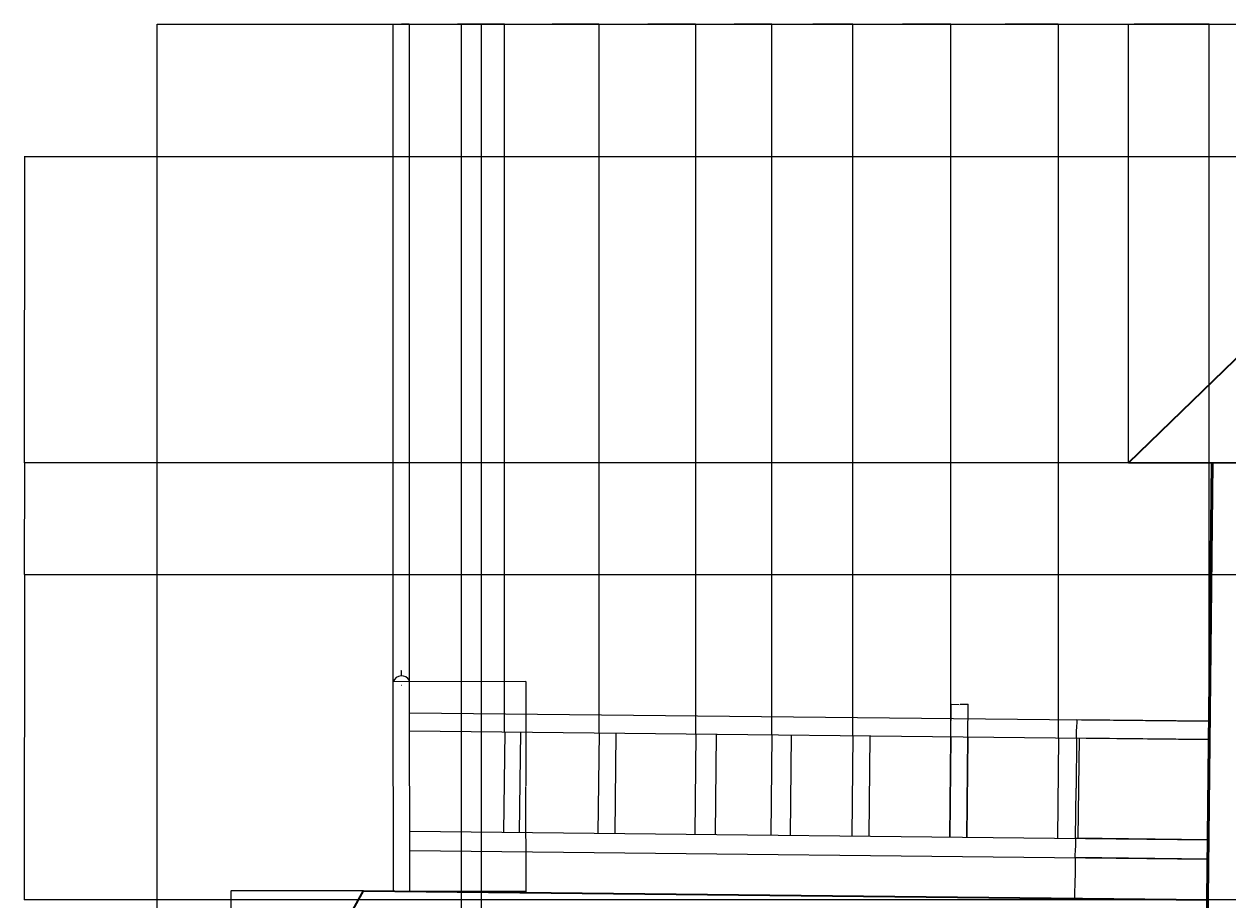
# Model space of a CAD drawing. Units: millimetres. Extents: x 1119 to 4262, y 854 to 2737.
# Tile 2 of 5: x 1119 to 2434, y 1780 to 2737. Entities that reach past the tile are written whole.
import ezdxf

# ---------------------------------------------------------------- set-up
doc = ezdxf.new("R2010")
doc.units = ezdxf.units.MM
for name, color, linetype, lineweight in [('A-ANNO-DIMS', 2, 'Continuous', 18), ('A-FLOR-HRAL', 5, 'Continuous', 18), ('A-ROOF', 1, 'Continuous', 35), ('A-WALL', 7, 'Continuous', 50)]:
    doc.layers.add(name, color=color, linetype=linetype, lineweight=lineweight)
doc.styles.get("Standard").update_dxf_attribs({"font": 'arial.ttf'})
doc.dimstyles.get("Standard").update_dxf_attribs({"dimtxt": 0.18, "dimasz": 0.18, "dimexe": 0.18, "dimexo": 0.0625, "dimgap": 0.09, "dimtad": 0, "dimtih": 1, "dimtoh": 1, "dimdec": 4, "dimzin": 0, "dimdsep": 46, "dimtxsty": 'Standard', "dimcen": 0.09, "dimadec": 0, "dimazin": 0, "dimtfac": 1, "dimtdec": 4, "dimtofl": 0, "dimtmove": 0, "dimatfit": 3, "dimfxl": 1, "dimtolj": 1, "dimtzin": 0, "dimarcsym": 0})

# ---------------------------------------------------------------- blocks, each defined once
blk = doc.blocks.new('*D13')
at = {"layer": 'A-ANNO-DIMS', "color": 0, "lineweight": -2, "transparency": 16777216}
for p, q in [((1264.4, 1028.3), (1264.4, 2737.1)), ((1264.5, 2737), (2690.1, 2737)), ((4116.6, 2737), (2691, 2737)), ((4116.8, 2249.8), (4116.8, 2737.1))]:
    blk.add_line(p, q, dxfattribs=at)
at = {"layer": 'A-ANNO-DIMS', "color": 0, "transparency": 16777216}
for points in [[(1264.5, 2737), (1264.5, 2736.9), (1264.4, 2737)], [(4116.6, 2737), (4116.6, 2736.9), (4116.8, 2737)]]:
    blk.add_solid(points, dxfattribs=at)
at = {"layer": 'Defpoints', "color": 0, "transparency": 16777216}
for p in [(4116.8, 2737), (4116.8, 2249.7), (1264.4, 1028.2)]:
    blk.add_point(p, dxfattribs=at)
at = {"layer": 'A-ANNO-DIMS', "color": 0, "transparency": 16777216, "insert": (2690.6, 2737), "char_height": 0.18, "attachment_point": 5}
blk.add_mtext('\\A1;2852.4', dxfattribs=at)
blk = doc.blocks.new('*D14')
at = {"layer": 'A-ANNO-DIMS', "color": 0, "lineweight": -2, "transparency": 16777216}
for p, q in [((2325.6, 2257.9), (2325.6, 2737.1)), ((2325.8, 2737), (2497.3, 2737)), ((2669.4, 2737), (2497.9, 2737)), ((2669.6, 2592), (2669.6, 2737.1))]:
    blk.add_line(p, q, dxfattribs=at)
at = {"layer": 'A-ANNO-DIMS', "color": 0, "transparency": 16777216}
for points in [[(2325.8, 2737), (2325.8, 2736.9), (2325.6, 2737)], [(2669.4, 2737), (2669.4, 2736.9), (2669.6, 2737)]]:
    blk.add_solid(points, dxfattribs=at)
at = {"layer": 'Defpoints', "color": 0, "transparency": 16777216}
for p in [(2669.6, 2737), (2669.6, 2592), (2325.6, 2257.9)]:
    blk.add_point(p, dxfattribs=at)
at = {"layer": 'A-ANNO-DIMS', "color": 0, "transparency": 16777216, "insert": (2497.6, 2737), "char_height": 0.18, "attachment_point": 5}
blk.add_mtext('\\A1;344', dxfattribs=at)
blk = doc.blocks.new('*D34')
at = {"layer": 'A-ANNO-DIMS', "color": 0, "lineweight": -2, "transparency": 16777216}
for p, q in [((2537.1, 2135.5), (1119.2, 2135.5)), ((1119.4, 2135.3), (1119.4, 1958.1)), ((1119.4, 1780.5), (1119.4, 1957.7)), ((2537.1, 1780.3), (1119.2, 1780.3))]:
    blk.add_line(p, q, dxfattribs=at)
at = {"layer": 'A-ANNO-DIMS', "color": 0, "transparency": 16777216}
for points in [[(1119.3, 2135.3), (1119.4, 2135.3), (1119.4, 2135.5)], [(1119.3, 1780.5), (1119.4, 1780.5), (1119.4, 1780.3)]]:
    blk.add_solid(points, dxfattribs=at)
at = {"layer": 'Defpoints', "color": 0, "transparency": 16777216}
for p in [(1119.4, 2135.5), (2537.2, 2135.5), (2537.2, 1780.3)]:
    blk.add_point(p, dxfattribs=at)
at = {"layer": 'A-ANNO-DIMS', "color": 0, "transparency": 16777216, "insert": (1119.4, 1957.9), "char_height": 0.18, "attachment_point": 5}
blk.add_mtext('\\A1;355.2', dxfattribs=at)
blk = doc.blocks.new('*D35')
at = {"layer": 'A-ANNO-DIMS', "color": 0, "lineweight": -2, "transparency": 16777216}
for p, q in [((2416.9, 2257.7), (1119.2, 2257.7)), ((1119.4, 2257.5), (1119.4, 2196.8)), ((1119.4, 2135.7), (1119.4, 2196.4)), ((2537.1, 2135.5), (1119.2, 2135.5))]:
    blk.add_line(p, q, dxfattribs=at)
at = {"layer": 'A-ANNO-DIMS', "color": 0, "transparency": 16777216}
for points in [[(1119.3, 2257.5), (1119.4, 2257.5), (1119.4, 2257.7)], [(1119.3, 2135.7), (1119.4, 2135.7), (1119.4, 2135.5)]]:
    blk.add_solid(points, dxfattribs=at)
at = {"layer": 'Defpoints', "color": 0, "transparency": 16777216}
for p in [(1119.4, 2257.7), (2417, 2257.7), (2537.2, 2135.5)]:
    blk.add_point(p, dxfattribs=at)
at = {"layer": 'A-ANNO-DIMS', "color": 0, "transparency": 16777216, "insert": (1119.4, 2196.6), "char_height": 0.18, "attachment_point": 5}
blk.add_mtext('\\A1;122.15', dxfattribs=at)
blk = doc.blocks.new('*D36')
at = {"layer": 'A-ANNO-DIMS', "color": 0, "lineweight": -2, "transparency": 16777216}
for p, q in [((2669.5, 2592), (1119.2, 2592)), ((1119.4, 2591.8), (1119.4, 2425)), ((1119.4, 2257.8), (1119.4, 2424.6)), ((2416.9, 2257.7), (1119.2, 2257.7))]:
    blk.add_line(p, q, dxfattribs=at)
at = {"layer": 'A-ANNO-DIMS', "color": 0, "transparency": 16777216}
for points in [[(1119.3, 2591.8), (1119.4, 2591.8), (1119.4, 2592)], [(1119.3, 2257.8), (1119.4, 2257.8), (1119.4, 2257.7)]]:
    blk.add_solid(points, dxfattribs=at)
at = {"layer": 'Defpoints', "color": 0, "transparency": 16777216}
for p in [(1119.4, 2592), (2669.6, 2592), (2417, 2257.7)]:
    blk.add_point(p, dxfattribs=at)
at = {"layer": 'A-ANNO-DIMS', "color": 0, "transparency": 16777216, "insert": (1119.4, 2424.8), "char_height": 0.18, "attachment_point": 5}
blk.add_mtext('\\A1;334.3', dxfattribs=at)
blk = doc.blocks.new('*D46')
at = {"layer": 'A-ANNO-DIMS', "color": 0, "lineweight": -2, "transparency": 16777216}
for p, q in [((1489.8, 1790.1), (1344.7, 1790.2)), ((1344.9, 1790), (1344.8, 1673.7)), ((1344.8, 1556.9), (1344.8, 1673.3)), ((1489.7, 1556.7), (1344.6, 1556.8))]:
    blk.add_line(p, q, dxfattribs=at)
at = {"layer": 'A-ANNO-DIMS', "color": 0, "transparency": 16777216}
for points in [[(1344.8, 1790), (1344.9, 1790), (1344.9, 1790.2)], [(1344.7, 1556.9), (1344.8, 1556.9), (1344.8, 1556.8)]]:
    blk.add_solid(points, dxfattribs=at)
at = {"layer": 'Defpoints', "color": 0, "transparency": 16777216}
for p in [(1344.9, 1790.2), (1489.9, 1790.1), (1489.8, 1556.7)]:
    blk.add_point(p, dxfattribs=at)
at = {"layer": 'A-ANNO-DIMS', "color": 0, "transparency": 16777216, "insert": (1344.8, 1673.5), "char_height": 0.18, "attachment_point": 5}
blk.add_mtext('\\A1;233.4', dxfattribs=at)
blk = doc.blocks.new('*D47')
at = {"layer": 'A-ANNO-DIMS', "color": 0, "lineweight": -2, "transparency": 16777216}
for p, q in [((1522.1, 2018.9), (1522.1, 2737.1)), ((1522.3, 2737), (1530.7, 2737)), ((1539.8, 2737), (1531.4, 2737)), ((1540, 2020.3), (1540, 2737.1))]:
    blk.add_line(p, q, dxfattribs=at)
at = {"layer": 'A-ANNO-DIMS', "color": 0, "transparency": 16777216}
for points in [[(1522.3, 2737), (1522.3, 2736.9), (1522.1, 2737)], [(1539.8, 2737), (1539.8, 2736.9), (1540, 2737)]]:
    blk.add_solid(points, dxfattribs=at)
at = {"layer": 'Defpoints', "color": 0, "transparency": 16777216}
for p in [(1540, 2737), (1522.1, 2018.9), (1540, 2020.2)]:
    blk.add_point(p, dxfattribs=at)
at = {"layer": 'A-ANNO-DIMS', "color": 0, "transparency": 16777216, "insert": (1531.1, 2737), "char_height": 0.18, "attachment_point": 5}
blk.add_mtext('\\A1;17.91', dxfattribs=at)
blk = doc.blocks.new('*D48')
at = {"layer": 'A-ANNO-DIMS', "color": 0, "lineweight": -2, "transparency": 16777216}
for p, q in [((1522.2, 2018.9), (1667.3, 2019.2)), ((1667.1, 2019), (1667.3, 1904.8)), ((1667.6, 1790.2), (1667.3, 1904.4)), ((1522.6, 1789.8), (1667.7, 1790))]:
    blk.add_line(p, q, dxfattribs=at)
at = {"layer": 'A-ANNO-DIMS', "color": 0, "transparency": 16777216}
for points in [[(1667.1, 2019), (1667.1, 2019), (1667.1, 2019.2)], [(1667.6, 1790.2), (1667.5, 1790.2), (1667.6, 1790)]]:
    blk.add_solid(points, dxfattribs=at)
at = {"layer": 'Defpoints', "color": 0, "transparency": 16777216}
for p in [(1522.1, 2018.9), (1522.6, 1789.8), (1667.6, 1790)]:
    blk.add_point(p, dxfattribs=at)
at = {"layer": 'A-ANNO-DIMS', "color": 0, "transparency": 16777216, "insert": (1667.3, 1904.6), "char_height": 0.18, "attachment_point": 5}
blk.add_mtext('\\A1;229.1', dxfattribs=at)
blk = doc.blocks.new('*D49')
at = {"layer": 'A-ANNO-DIMS', "color": 0, "lineweight": -2, "transparency": 16777216}
for p, q in [((2412.4, 1825), (2267.2, 1826.5)), ((2267.4, 1826.4), (2267.2, 1804.4)), ((2267, 1782.1), (2267.2, 1804.1)), ((2411.9, 1780.4), (2266.8, 1781.9))]:
    blk.add_line(p, q, dxfattribs=at)
at = {"layer": 'A-ANNO-DIMS', "color": 0, "transparency": 16777216}
for points in [[(2267.4, 1826.4), (2267.5, 1826.4), (2267.4, 1826.5)], [(2266.9, 1782.1), (2267, 1782.1), (2267, 1781.9)]]:
    blk.add_solid(points, dxfattribs=at)
at = {"layer": 'Defpoints', "color": 0, "transparency": 16777216}
for p in [(2267.4, 1826.5), (2412.4, 1825), (2411.9, 1780.4)]:
    blk.add_point(p, dxfattribs=at)
at = {"layer": 'A-ANNO-DIMS', "color": 0, "transparency": 16777216, "insert": (2267.2, 1804.2), "char_height": 0.18, "attachment_point": 5}
blk.add_mtext('\\A1;44.63', dxfattribs=at)
blk = doc.blocks.new('*D50')
at = {"layer": 'A-ANNO-DIMS', "color": 0, "lineweight": -2, "transparency": 16777216}
for p, q in [((2412.6, 1846.1), (2267.5, 1847.7)), ((2267.6, 1847.5), (2267.5, 1837.3)), ((2267.4, 1826.7), (2267.5, 1836.9)), ((2412.4, 1825), (2267.2, 1826.5))]:
    blk.add_line(p, q, dxfattribs=at)
at = {"layer": 'A-ANNO-DIMS', "color": 0, "transparency": 16777216}
for points in [[(2267.6, 1847.5), (2267.7, 1847.5), (2267.7, 1847.7)], [(2267.4, 1826.7), (2267.5, 1826.7), (2267.4, 1826.5)]]:
    blk.add_solid(points, dxfattribs=at)
at = {"layer": 'Defpoints', "color": 0, "transparency": 16777216}
for p in [(2267.7, 1847.7), (2412.6, 1846.1), (2412.4, 1825)]:
    blk.add_point(p, dxfattribs=at)
at = {"layer": 'A-ANNO-DIMS', "color": 0, "transparency": 16777216, "insert": (2267.5, 1837.1), "char_height": 0.18, "attachment_point": 5}
blk.add_mtext('\\A1;21.117', dxfattribs=at)
blk = doc.blocks.new('*D51')
at = {"layer": 'A-ANNO-DIMS', "color": 0, "lineweight": -2, "transparency": 16777216}
for p, q in [((2268.8, 1957), (2268.2, 1902.6)), ((2413.7, 1955.7), (2268.6, 1957.2)), ((2267.7, 1847.8), (2268.2, 1902.3)), ((2412.6, 1846.1), (2267.5, 1847.7))]:
    blk.add_line(p, q, dxfattribs=at)
at = {"layer": 'A-ANNO-DIMS', "color": 0, "transparency": 16777216}
for points in [[(2268.8, 1957), (2268.8, 1957), (2268.8, 1957.2)], [(2267.6, 1847.8), (2267.7, 1847.8), (2267.7, 1847.7)]]:
    blk.add_solid(points, dxfattribs=at)
at = {"layer": 'Defpoints', "color": 0, "transparency": 16777216}
for p in [(2268.8, 1957.2), (2413.8, 1955.7), (2412.6, 1846.1)]:
    blk.add_point(p, dxfattribs=at)
at = {"layer": 'A-ANNO-DIMS', "color": 0, "transparency": 16777216, "insert": (2268.2, 1902.4), "char_height": 0.18, "attachment_point": 5}
blk.add_mtext('\\A1;109.56', dxfattribs=at)
blk = doc.blocks.new('*D52')
at = {"layer": 'A-ANNO-DIMS', "color": 0, "lineweight": -2, "transparency": 16777216}
for p, q in [((2413.9, 1975.5), (2268.8, 1977)), ((2269, 1976.8), (2268.9, 1967.3)), ((2268.8, 1957.4), (2268.9, 1966.9)), ((2413.7, 1955.7), (2268.6, 1957.2))]:
    blk.add_line(p, q, dxfattribs=at)
at = {"layer": 'A-ANNO-DIMS', "color": 0, "transparency": 16777216}
for points in [[(2269, 1976.8), (2269, 1976.8), (2269, 1977)], [(2268.8, 1957.4), (2268.8, 1957.4), (2268.8, 1957.2)]]:
    blk.add_solid(points, dxfattribs=at)
at = {"layer": 'Defpoints', "color": 0, "transparency": 16777216}
for p in [(2269, 1977), (2414, 1975.5), (2413.8, 1955.7)]:
    blk.add_point(p, dxfattribs=at)
at = {"layer": 'A-ANNO-DIMS', "color": 0, "transparency": 16777216, "insert": (2268.9, 1967.1), "char_height": 0.18, "attachment_point": 5}
blk.add_mtext('\\A1;19.8', dxfattribs=at)
blk = doc.blocks.new('*D53')
at = {"layer": 'A-ANNO-DIMS', "color": 0, "lineweight": -2, "transparency": 16777216}
for p, q in [((1540.1, 1965), (1540.1, 2737.1)), ((1540.3, 2737), (1591.6, 2737)), ((1643.9, 2737), (1592.5, 2737)), ((1644, 1963.9), (1644, 2737.1))]:
    blk.add_line(p, q, dxfattribs=at)
at = {"layer": 'A-ANNO-DIMS', "color": 0, "transparency": 16777216}
for points in [[(1540.3, 2737), (1540.3, 2736.9), (1540.1, 2737)], [(1643.9, 2737), (1643.9, 2736.9), (1644, 2737)]]:
    blk.add_solid(points, dxfattribs=at)
at = {"layer": 'Defpoints', "color": 0, "transparency": 16777216}
for p in [(1644, 2737), (1540.1, 1964.9), (1644, 1963.8)]:
    blk.add_point(p, dxfattribs=at)
at = {"layer": 'A-ANNO-DIMS', "color": 0, "transparency": 16777216, "insert": (1592.1, 2737), "char_height": 0.18, "attachment_point": 5}
blk.add_mtext('\\A1;103.92', dxfattribs=at)
blk = doc.blocks.new('*D54')
at = {"layer": 'A-ANNO-DIMS', "color": 0, "lineweight": -2, "transparency": 16777216}
for p, q in [((1644, 1963.9), (1644, 2737.1)), ((1644.2, 2737), (1695.1, 2737)), ((1746.9, 2737), (1696, 2737)), ((1747.1, 1962.8), (1747.1, 2737.1))]:
    blk.add_line(p, q, dxfattribs=at)
at = {"layer": 'A-ANNO-DIMS', "color": 0, "transparency": 16777216}
for points in [[(1644.2, 2737), (1644.2, 2736.9), (1644, 2737)], [(1746.9, 2737), (1746.9, 2736.9), (1747.1, 2737)]]:
    blk.add_solid(points, dxfattribs=at)
at = {"layer": 'Defpoints', "color": 0, "transparency": 16777216}
for p in [(1747.1, 2737), (1644, 1963.8), (1747.1, 1962.7)]:
    blk.add_point(p, dxfattribs=at)
at = {"layer": 'A-ANNO-DIMS', "color": 0, "transparency": 16777216, "insert": (1695.6, 2737), "char_height": 0.18, "attachment_point": 5}
blk.add_mtext('\\A1;103.05', dxfattribs=at)
blk = doc.blocks.new('*D55')
at = {"layer": 'A-ANNO-DIMS', "color": 0, "lineweight": -2, "transparency": 16777216}
for p, q in [((1747.1, 1962.8), (1747.1, 2737.1)), ((1747.3, 2737), (1799.5, 2737)), ((1852.6, 2737), (1800.4, 2737)), ((1852.8, 1961.7), (1852.8, 2737.1))]:
    blk.add_line(p, q, dxfattribs=at)
at = {"layer": 'A-ANNO-DIMS', "color": 0, "transparency": 16777216}
for points in [[(1747.3, 2737), (1747.3, 2736.9), (1747.1, 2737)], [(1852.6, 2737), (1852.6, 2736.9), (1852.8, 2737)]]:
    blk.add_solid(points, dxfattribs=at)
at = {"layer": 'Defpoints', "color": 0, "transparency": 16777216}
for p in [(1852.8, 2737), (1747.1, 1962.7), (1852.8, 1961.6)]:
    blk.add_point(p, dxfattribs=at)
at = {"layer": 'A-ANNO-DIMS', "color": 0, "transparency": 16777216, "insert": (1799.9, 2737), "char_height": 0.18, "attachment_point": 5}
blk.add_mtext('\\A1;105.67', dxfattribs=at)
blk = doc.blocks.new('*D56')
at = {"layer": 'A-ANNO-DIMS', "color": 0, "lineweight": -2, "transparency": 16777216}
for p, q in [((1852.8, 1961.7), (1852.8, 2737.1)), ((1852.9, 2737), (1894, 2737)), ((1935.8, 2737), (1894.7, 2737)), ((1936, 1960.8), (1936, 2737.1))]:
    blk.add_line(p, q, dxfattribs=at)
at = {"layer": 'A-ANNO-DIMS', "color": 0, "transparency": 16777216}
for points in [[(1852.9, 2737), (1852.9, 2736.9), (1852.8, 2737)], [(1935.8, 2737), (1935.8, 2736.9), (1936, 2737)]]:
    blk.add_solid(points, dxfattribs=at)
at = {"layer": 'Defpoints', "color": 0, "transparency": 16777216}
for p in [(1936, 2737), (1852.8, 1961.6), (1936, 1960.7)]:
    blk.add_point(p, dxfattribs=at)
at = {"layer": 'A-ANNO-DIMS', "color": 0, "transparency": 16777216, "insert": (1894.4, 2737), "char_height": 0.18, "attachment_point": 5}
blk.add_mtext('\\A1;83.2', dxfattribs=at)
blk = doc.blocks.new('*D57')
at = {"layer": 'A-ANNO-DIMS', "color": 0, "lineweight": -2, "transparency": 16777216}
for p, q in [((1936, 1960.8), (1936, 2737.1)), ((1936.2, 2737), (1979.8, 2737)), ((2024.3, 2737), (1980.6, 2737)), ((2024.5, 1959.9), (2024.5, 2737.1))]:
    blk.add_line(p, q, dxfattribs=at)
at = {"layer": 'A-ANNO-DIMS', "color": 0, "transparency": 16777216}
for points in [[(1936.2, 2737), (1936.2, 2736.9), (1936, 2737)], [(2024.3, 2737), (2024.3, 2736.9), (2024.5, 2737)]]:
    blk.add_solid(points, dxfattribs=at)
at = {"layer": 'Defpoints', "color": 0, "transparency": 16777216}
for p in [(2024.5, 2737), (1936, 1960.7), (2024.5, 1959.8)]:
    blk.add_point(p, dxfattribs=at)
at = {"layer": 'A-ANNO-DIMS', "color": 0, "transparency": 16777216, "insert": (1980.2, 2737), "char_height": 0.18, "attachment_point": 5}
blk.add_mtext('\\A1;88.52', dxfattribs=at)
blk = doc.blocks.new('*D58')
at = {"layer": 'A-ANNO-DIMS', "color": 0, "lineweight": -2, "transparency": 16777216}
for p, q in [((2024.5, 1959.9), (2024.5, 2737.1)), ((2024.7, 2737), (2077.5, 2737)), ((2131.3, 2737), (2078.5, 2737)), ((2131.5, 1958.7), (2131.5, 2737.1))]:
    blk.add_line(p, q, dxfattribs=at)
at = {"layer": 'A-ANNO-DIMS', "color": 0, "transparency": 16777216}
for points in [[(2024.7, 2737), (2024.7, 2736.9), (2024.5, 2737)], [(2131.3, 2737), (2131.3, 2736.9), (2131.5, 2737)]]:
    blk.add_solid(points, dxfattribs=at)
at = {"layer": 'Defpoints', "color": 0, "transparency": 16777216}
for p in [(2131.5, 2737), (2024.5, 1959.8), (2131.5, 1958.7)]:
    blk.add_point(p, dxfattribs=at)
at = {"layer": 'A-ANNO-DIMS', "color": 0, "transparency": 16777216, "insert": (2078, 2737), "char_height": 0.18, "attachment_point": 5}
blk.add_mtext('\\A1;107.04', dxfattribs=at)
blk = doc.blocks.new('*D59')
at = {"layer": 'A-ANNO-DIMS', "color": 0, "lineweight": -2, "transparency": 16777216}
for p, q in [((2131.5, 1958.7), (2131.5, 2737.1)), ((2131.7, 2737), (2189.8, 2737)), ((2248.8, 2737), (2190.7, 2737)), ((2249, 1957.5), (2249, 2737.1))]:
    blk.add_line(p, q, dxfattribs=at)
at = {"layer": 'A-ANNO-DIMS', "color": 0, "transparency": 16777216}
for points in [[(2131.7, 2737), (2131.7, 2736.9), (2131.5, 2737)], [(2248.8, 2737), (2248.8, 2736.9), (2249, 2737)]]:
    blk.add_solid(points, dxfattribs=at)
at = {"layer": 'Defpoints', "color": 0, "transparency": 16777216}
for p in [(2249, 2737), (2131.5, 1958.7), (2249, 1957.4)]:
    blk.add_point(p, dxfattribs=at)
at = {"layer": 'A-ANNO-DIMS', "color": 0, "transparency": 16777216, "insert": (2190.3, 2737), "char_height": 0.18, "attachment_point": 5}
blk.add_mtext('\\A1;117.48', dxfattribs=at)
blk = doc.blocks.new('*D60')
at = {"layer": 'A-ANNO-DIMS', "color": 0, "lineweight": -2, "transparency": 16777216}
for p, q in [((2249, 1957.5), (2249, 2737.1)), ((2249.2, 2737), (2331, 2737)), ((2413.6, 2737), (2331.8, 2737)), ((2413.8, 1955.8), (2413.8, 2737.1))]:
    blk.add_line(p, q, dxfattribs=at)
at = {"layer": 'A-ANNO-DIMS', "color": 0, "transparency": 16777216}
for points in [[(2249.2, 2737), (2249.2, 2736.9), (2249, 2737)], [(2413.6, 2737), (2413.6, 2736.9), (2413.8, 2737)]]:
    blk.add_solid(points, dxfattribs=at)
at = {"layer": 'Defpoints', "color": 0, "transparency": 16777216}
for p in [(2413.8, 2737), (2249, 1957.4), (2413.8, 1955.7)]:
    blk.add_point(p, dxfattribs=at)
at = {"layer": 'A-ANNO-DIMS', "color": 0, "transparency": 16777216, "insert": (2331.4, 2737), "char_height": 0.18, "attachment_point": 5}
blk.add_mtext('\\A1;164.8', dxfattribs=at)
blk = doc.blocks.new('*D61')
at = {"layer": 'A-ANNO-DIMS', "color": 0, "lineweight": -2, "transparency": 16777216}
for p, q in [((2130.4, 1849.2), (2131.9, 1994.3)), ((2132.1, 1994.1), (2140.7, 1994)), ((2150.2, 1993.9), (2141.6, 1994)), ((2148.8, 1849), (2150.4, 1994.1))]:
    blk.add_line(p, q, dxfattribs=at)
at = {"layer": 'A-ANNO-DIMS', "color": 0, "transparency": 16777216}
for points in [[(2132.1, 1994.1), (2132.1, 1994.1), (2131.9, 1994.1)], [(2150.2, 1993.9), (2150.2, 1993.9), (2150.4, 1993.9)]]:
    blk.add_solid(points, dxfattribs=at)
at = {"layer": 'Defpoints', "color": 0, "transparency": 16777216}
for p in [(2150.4, 1993.9), (2130.4, 1849.1), (2148.8, 1848.9)]:
    blk.add_point(p, dxfattribs=at)
at = {"layer": 'A-ANNO-DIMS', "color": 0, "transparency": 16777216, "insert": (2141.1, 1994), "char_height": 0.18, "attachment_point": 5}
blk.add_mtext('\\A1;18.466', dxfattribs=at)
blk = doc.blocks.new('*D79')
at = {"layer": 'A-ANNO-DIMS', "color": 0, "lineweight": -2, "transparency": 16777216}
for p, q in [((1596.9, 1456), (1596.9, 2737.1)), ((1597.1, 2737), (1607.4, 2737)), ((1618.6, 2737), (1608.3, 2737)), ((1618.7, 1432.9), (1618.7, 2737.1))]:
    blk.add_line(p, q, dxfattribs=at)
at = {"layer": 'A-ANNO-DIMS', "color": 0, "transparency": 16777216}
for points in [[(1597.1, 2737), (1597.1, 2736.9), (1596.9, 2737)], [(1618.6, 2737), (1618.6, 2736.9), (1618.7, 2737)]]:
    blk.add_solid(points, dxfattribs=at)
at = {"layer": 'Defpoints', "color": 0, "transparency": 16777216}
for p in [(1618.7, 2737), (1596.9, 1455.9), (1618.7, 1432.9)]:
    blk.add_point(p, dxfattribs=at)
at = {"layer": 'A-ANNO-DIMS', "color": 0, "transparency": 16777216, "insert": (1607.8, 2737), "char_height": 0.18, "attachment_point": 5}
blk.add_mtext('\\A1;21.813', dxfattribs=at)
blk = doc.blocks.new('*D90')
at = {"layer": 'A-ANNO-DIMS', "color": 0, "lineweight": -2, "transparency": 16777216}
for p, q in [((1530.6, 2031.1), (1530.8, 2031.1)), ((1530.8, 2031.1), (1531, 2025.2)), ((1531.3, 2014.9), (1531.5, 2014.9)), ((1531.4, 2014.8), (1531.4, 2015))]:
    blk.add_line(p, q, dxfattribs=at)
at = {"layer": 'A-ANNO-DIMS', "color": 0, "transparency": 16777216}
blk.add_solid([(1531, 2025.2), (1531, 2025.2), (1531, 2025)], dxfattribs=at)
at = {"layer": 'Defpoints', "color": 0, "transparency": 16777216}
for p in [(1531, 2025), (1531.4, 2014.9)]:
    blk.add_point(p, dxfattribs=at)
at = {"layer": 'A-ANNO-DIMS', "color": 0, "transparency": 16777216, "insert": (1530, 2031.1), "char_height": 0.18, "attachment_point": 5}
blk.add_mtext('\\A1;R10.102', dxfattribs=at)

msp = doc.modelspace()

# ---------------------------------------------------------------- linework, layer by layer
at = {"layer": 'A-FLOR-HRAL'}
for p, q in [((1522.551, 1789.7652), (1522.1092, 2018.8871)), ((1540.4627, 1789.5764), (1540.018, 2020.188)), ((1540.0864, 1984.7036), (2414.0059, 1975.4907)), ((1540.1246, 1964.9025), (2413.7972, 1955.6923)), ((1644.0493, 1963.807), (1642.8943, 1854.2491)), ((1661.1516, 1963.6267), (1659.9966, 1854.0688)), ((1747.0945, 1962.7207), (1745.9396, 1853.1628)), ((1765.5177, 1962.5265), (1764.3628, 1852.9686)), ((1852.7676, 1961.6067), (1851.6126, 1852.0488)), ((1875.1953, 1961.3702), (1874.0404, 1851.8124)), ((1935.9713, 1960.7295), (1934.8163, 1851.1717)), ((1957.1198, 1960.5066), (1955.9648, 1850.9487)), ((2024.4864, 1959.7964), (2023.3315, 1850.2385)), ((2042.9096, 1959.6022), (2041.7547, 1850.0443)), ((2131.5222, 1958.668), (2130.3672, 1849.1102)), ((2149.9871, 1958.4734), (2148.8322, 1848.9155)), ((2249, 1957.4296), (2247.845, 1847.8717)), ((2271.5251, 1957.1921), (2270.3702, 1847.6343)), ((1540.3359, 1855.3303), (2412.6422, 1846.1344)), ((1540.3766, 1834.2116), (2412.4196, 1825.0185))]:
    msp.add_line(p, q, dxfattribs=at)
msp.add_arc((1531.399, 2014.9196), 10.1016, 31.4355131, 156.8738456, dxfattribs=at)
at = {"layer": 'A-ROOF'}
for p, q in [((2325.6262, 2257.8652), (2669.6107, 2591.9672)), ((3323.0337, 2255.5648), (2325.6262, 2257.8652)), ((1360.1359, 1558.0571), (1489.8677, 1790.1098)), ((1489.8677, 1790.1098), (2411.9491, 1780.3892))]:
    msp.add_line(p, q, dxfattribs=at)
at = {"layer": 'A-WALL'}
msp.add_line((2416.9805, 2257.6545), (2403.8929, 1016.1891), dxfattribs=at)

# ---------------------------------------------------------------- dimensions: what is measured, and where the dimension line sits
at = {"layer": 'A-ANNO-DIMS'}
for base, p1, p2, override, picture, middle in [((4116.7957, 2736.9672), (1264.3595, 1028.2021), (4116.7957, 2249.7378), {"dimdec": 1, "dimlfac": 1, "dimrnd": 0, "dimzin": 0, "dimdsep": 46, "dimlunit": 2}, '*D13', (2690.5776, 2736.9672)), ((1540.018, 2736.9672), (1522.1092, 2018.8871), (1540.018, 2020.188), {"dimdec": 2, "dimlfac": 1, "dimrnd": 0, "dimzin": 0, "dimdsep": 46, "dimlunit": 2}, '*D47', (1531.0636, 2736.9672)), ((1644.0493, 2736.9672), (1540.1246, 1964.9025), (1644.0493, 1963.807), {"dimdec": 2, "dimlfac": 1, "dimrnd": 0, "dimzin": 0, "dimdsep": 46, "dimlunit": 2}, '*D53', (1592.0869, 2736.9672)), ((1618.74978, 2736.96722), (1596.93635, 1455.94989), (1618.74978, 1432.86755), {"dimdec": 3, "dimlfac": 1, "dimrnd": 0, "dimzin": 0, "dimdsep": 46, "dimlunit": 2}, '*D79', (1607.84307, 2736.96722)), ((1747.0945, 2736.9672), (1644.0493, 1963.807), (1747.0945, 1962.7207), {"dimdec": 2, "dimlfac": 1, "dimrnd": 0, "dimzin": 0, "dimdsep": 46, "dimlunit": 2}, '*D54', (1695.5719, 2736.9672)), ((1852.7676, 2736.9672), (1747.0945, 1962.7207), (1852.7676, 1961.6067), {"dimdec": 2, "dimlfac": 1, "dimrnd": 0, "dimzin": 0, "dimdsep": 46, "dimlunit": 2}, '*D55', (1799.9311, 2736.9672)), ((1935.9713, 2736.9672), (1852.7676, 1961.6067), (1935.9713, 1960.7295), {"dimdec": 1, "dimlfac": 1, "dimrnd": 0, "dimzin": 0, "dimdsep": 46, "dimlunit": 2}, '*D56', (1894.3694, 2736.9672)), ((2024.4864, 2736.9672), (1935.9713, 1960.7295), (2024.4864, 1959.7964), {"dimdec": 2, "dimlfac": 1, "dimrnd": 0, "dimzin": 0, "dimdsep": 46, "dimlunit": 2}, '*D57', (1980.2288, 2736.9672)), ((2131.5222, 2736.9672), (2024.4864, 1959.7964), (2131.5222, 1958.668), {"dimdec": 2, "dimlfac": 1, "dimrnd": 0, "dimzin": 0, "dimdsep": 46, "dimlunit": 2}, '*D58', (2078.0043, 2736.9672)), ((2249, 2736.9672), (2131.5222, 1958.668), (2249, 1957.4296), {"dimdec": 2, "dimlfac": 1, "dimrnd": 0, "dimzin": 0, "dimdsep": 46, "dimlunit": 2}, '*D59', (2190.2611, 2736.9672)), ((2413.7972, 2736.9672), (2249, 1957.4296), (2413.7972, 1955.6923), {"dimdec": 1, "dimlfac": 1, "dimrnd": 0, "dimzin": 0, "dimdsep": 46, "dimlunit": 2}, '*D60', (2331.3986, 2736.9672)), ((2669.6107, 2736.9672), (2325.6262, 2257.8652), (2669.6107, 2591.9672), {"dimdec": 0, "dimlfac": 1, "dimrnd": 0, "dimzin": 0, "dimdsep": 46, "dimlunit": 2}, '*D14', (2497.6185, 2736.9672))]:
    dim = msp.add_linear_dim(base=base, p1=p1, p2=p2, dimstyle='Standard', override=override, dxfattribs=at)
    dim.commit()
    dim.dimension.update_dxf_attribs({"geometry": picture, "text_midpoint": middle})
for base, p1, p2, angle, override, picture, middle in [((1119.3595, 2591.9672), (2416.9805, 2257.6545), (2669.6107, 2591.9672), 90, {"dimdec": 1, "dimlfac": 1, "dimrnd": 0, "dimzin": 0, "dimdsep": 46, "dimlunit": 2}, '*D36', (1119.3595, 2424.8109)), ((1119.3595, 2257.6545), (2537.1892, 2135.5085), (2416.9805, 2257.6545), 90, {"dimdec": 2, "dimlfac": 1, "dimrnd": 0, "dimzin": 0, "dimdsep": 46, "dimlunit": 2}, '*D35', (1119.3595, 2196.5815)), ((1119.3595, 2135.5085), (2537.1892, 1780.2865), (2537.1892, 2135.5085), 90, {"dimdec": 1, "dimlfac": 1, "dimrnd": 0, "dimzin": 0, "dimdsep": 46, "dimlunit": 2}, '*D34', (1119.3595, 1957.8975)), ((1667.5508, 1790.0448), (1522.1092, 2018.8871), (1522.551, 1789.7652), 270.1104871, {"dimdec": 1, "dimlfac": 1, "dimrnd": 0, "dimzin": 0, "dimdsep": 46, "dimlunit": 2}, '*D48', (1667.3299, 1904.6058)), ((2150.3607, 1993.9075), (2130.3672, 1849.1102), (2148.8322, 1848.9155), 359.3960099, {"dimdec": 3, "dimlfac": 1, "dimrnd": 0, "dimzin": 0, "dimdsep": 46, "dimlunit": 2}, '*D61', (2141.1282, 1994.0048)), ((2269.014, 1977.0192), (2413.7972, 1955.6923), (2414.0059, 1975.4907), 89.3960099, {"dimdec": 1, "dimlfac": 1, "dimrnd": 0, "dimzin": 0, "dimdsep": 46, "dimlunit": 2}, '*D52', (2268.9096, 1967.12)), ((2268.8052, 1957.2208), (2412.6422, 1846.1344), (2413.7972, 1955.6923), 89.3960099, {"dimdec": 2, "dimlfac": 1, "dimrnd": 0, "dimzin": 0, "dimdsep": 46, "dimlunit": 2}, '*D51', (2268.2278, 1902.4419)), ((2267.6503, 1847.6629), (2412.4196, 1825.0185), (2412.6422, 1846.1344), 89.3960099, {"dimdec": 3, "dimlfac": 1, "dimrnd": 0, "dimzin": 0, "dimdsep": 46, "dimlunit": 2}, '*D50', (2267.539, 1837.105)), ((2267.4277, 1826.547), (2411.9491, 1780.3892), (2412.4196, 1825.0185), 89.3960099, {"dimdec": 2, "dimlfac": 1, "dimrnd": 0, "dimzin": 0, "dimdsep": 46, "dimlunit": 2}, '*D49', (2267.1924, 1804.2323)), ((1344.8677, 1790.1787), (1489.7567, 1556.6906), (1489.8677, 1790.1098), 89.9727569, {"dimdec": 1, "dimlfac": 1, "dimrnd": 0, "dimzin": 0, "dimdsep": 46, "dimlunit": 2}, '*D46', (1344.8122, 1673.4691))]:
    dim = msp.add_linear_dim(base=base, p1=p1, p2=p2, angle=angle, dimstyle='Standard', override=override, dxfattribs=at)
    dim.commit()
    dim.dimension.update_dxf_attribs({"geometry": picture, "text_midpoint": middle})
dim = msp.add_radius_dim(center=(1531.399, 2014.9196), mpoint=(1530.9995, 2025.0133), dimstyle='Standard', override={"dimdec": 3, "dimlfac": 1, "dimrnd": 0, "dimzin": 0, "dimdsep": 46, "dimlunit": 2}, dxfattribs=at)
dim.commit()
dim.dimension.update_dxf_attribs({"geometry": '*D90', "text_midpoint": (1530.0309, 2031.0695), "dimtype": 164})

doc.saveas('drawing.dxf')
